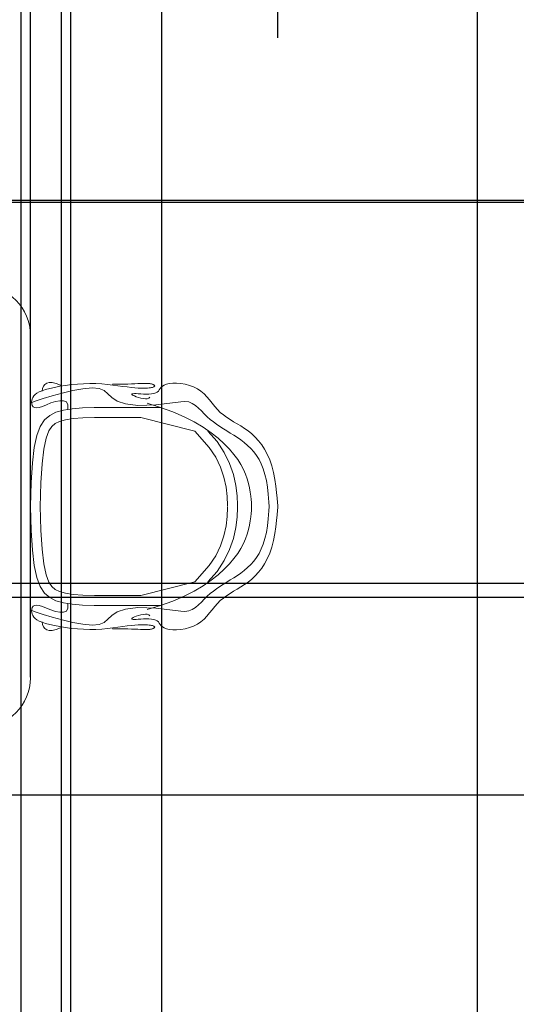
# Model space of a CAD drawing. Units: inches. Extents: x 1454 to 2136, y 626 to 1213.
# Tile 17 of 23: x 1701 to 1741, y 1062 to 1141. Entities that reach past the tile are written whole.
import ezdxf

# ---------------------------------------------------------------- set-up
doc = ezdxf.new("R2010")
doc.units = ezdxf.units.IN
doc.header["$MEASUREMENT"] = 0
for name, color, linetype, lineweight in [('A-ANNO-DIMS', 2, 'Continuous', 18), ('A-FURN-PATT', 252, 'Continuous', 13), ('conference', 41, 'Continuous', 18)]:
    doc.layers.add(name, color=color, linetype=linetype, lineweight=lineweight)
doc.styles.get("Standard").update_dxf_attribs({"font": 'arial.ttf'})
doc.dimstyles.get("Standard").update_dxf_attribs({"dimtxt": 4, "dimasz": 0.18, "dimexe": 0.18, "dimexo": 0.0625, "dimgap": 0.09, "dimtad": 0, "dimtih": 1, "dimtoh": 1, "dimdec": 0, "dimrnd": 6, "dimzin": 0, "dimdsep": 46, "dimlunit": 3, "dimtxsty": 'Standard', "dimcen": 0.09, "dimadec": 0, "dimazin": 0, "dimtfac": 1, "dimtdec": 0, "dimtofl": 0, "dimtmove": 0, "dimatfit": 3, "dimfxl": 1, "dimtolj": 1, "dimtzin": 0, "dimarcsym": 0})

# ---------------------------------------------------------------- blocks, each defined once
blk = doc.blocks.new('ОГ52_на12персон_стол2800х900')
for p, q in [((1400, 179.3), (1400, -520.7)), ((1433.5, 81.2), (1429.7, 78.7)), ((1438.5, 82.4), (1433.5, 81.2)), ((1444.8, 82.3), (1438.5, 82.4)), ((1452.5, 80.6), (1444.8, 82.3)), ((1461.7, 77.3), (1452.5, 80.6)), ((1629.1, 80.6), (1624.7, 80.4)), ((1633, 80.7), (1629.1, 80.6)), ((1636.3, 80.7), (1633, 80.7)), ((1639.2, 80.6), (1636.3, 80.7)), ((1641.7, 80.4), (1639.2, 80.6)), ((1643.8, 80.2), (1641.7, 80.4)), ((1683.8, 80.4), (1690.9, 81.1)), ((1690.9, 81.1), (1698.8, 81.1)), ((1698.8, 81.1), (1707.3, 80.4)), ((1409.5, 58), (1413.2, 60.6)), ((1413.2, 60.6), (1417.9, 63.2)), ((1417.9, 63.2), (1423.8, 65.6)), ((1425, 70.5), (1423.8, 65)), ((1423.8, 65.6), (1431, 68)), ((1426.9, 75.1), (1425, 70.5)), ((1429.7, 78.7), (1426.9, 75.1)), ((1431, 68), (1439.6, 70.4)), ((1439.6, 70.4), (1449.3, 72.6)), ((1465.2, 60.9), (1444.5, 55.2)), ((1449.3, 72.6), (1460.1, 74.7)), ((1460.1, 74.7), (1471.6, 76.5)), ((1486.6, 66), (1465.2, 60.9)), ((1471.6, 76.5), (1483.7, 78.1)), ((1483.7, 78.1), (1496.2, 79.3)), ((1507.4, 69.8), (1486.6, 66)), ((1496.2, 79.3), (1508.8, 80.1)), ((1526, 71.6), (1507.4, 69.8)), ((1508.8, 80.1), (1521.4, 80.4)), ((1521.4, 80.4), (1533.8, 80.2)), ((1540.7, 70.5), (1526, 71.6)), ((1533.8, 80.2), (1545.8, 79.5)), ((1550.8, 66.2), (1540.7, 70.5)), ((1545.8, 79.5), (1557.4, 78.6)), ((1558.5, 59.6), (1550.8, 66.2)), ((1557.4, 78.6), (1568.5, 77.3)), ((1579.5, 79.2), (1567.8, 79.4)), ((1568.5, 77.3), (1579, 76)), ((1579, 76), (1588.9, 74.6)), ((1589.9, 79.2), (1579.5, 79.2)), ((1588.9, 74.6), (1598, 73.4)), ((1598.9, 79.4), (1589.9, 79.2)), ((1598, 73.4), (1606.3, 72.3)), ((1606.8, 79.6), (1598.9, 79.4)), ((1606.3, 72.3), (1613.7, 71.5)), ((1613.7, 79.9), (1606.8, 79.6)), ((1619.6, 80.2), (1613.7, 79.9)), ((1613.7, 71.5), (1620.3, 71)), ((1624.7, 80.4), (1619.6, 80.2)), ((1620.3, 71), (1626.1, 70.7)), ((1626.1, 70.7), (1631.2, 70.7)), ((1631.2, 70.7), (1635.6, 70.7)), ((1635.6, 70.7), (1639.4, 71)), ((1639.4, 71), (1642.6, 71.3)), ((1642.6, 71.3), (1645.3, 71.7)), ((1645.6, 79.9), (1643.8, 80.2)), ((1645.3, 71.7), (1647.6, 72.1)), ((1647.2, 79.6), (1645.6, 79.9)), ((1648.6, 79.2), (1647.2, 79.6)), ((1647.6, 72.1), (1649.5, 72.6)), ((1649.8, 78.9), (1648.6, 79.2)), ((1649.5, 72.6), (1651, 73.1)), ((1650.9, 78.4), (1649.8, 78.9)), ((1651.8, 78), (1650.9, 78.4)), ((1651, 73.1), (1652.2, 73.6)), ((1652.6, 77.6), (1651.8, 78)), ((1652.2, 73.6), (1653, 74.1)), ((1652.2, 59.9), (1656.2, 61.1)), ((1653.2, 77.1), (1652.6, 77.6)), ((1653, 74.1), (1653.6, 74.6)), ((1653.6, 76.6), (1653.2, 77.1)), ((1653.9, 76.2), (1653.6, 76.6)), ((1653.6, 74.6), (1653.9, 75.1)), ((1654, 75.6), (1653.9, 76.2)), ((1653.9, 75.1), (1654, 75.6)), ((1656.2, 61.1), (1659.2, 62.9)), ((1659.2, 62.9), (1661.5, 65)), ((1661.5, 65), (1663.4, 67.5)), ((1663.4, 67.5), (1665.3, 70.1)), ((1665.3, 70.1), (1667.4, 72.7)), ((1667.4, 72.7), (1669.9, 75.2)), ((1669.9, 75.2), (1673.4, 77.4)), ((1673.4, 77.4), (1677.9, 79.2)), ((1677.9, 79.2), (1683.8, 80.4)), ((1707.3, 80.4), (1716.1, 78.9)), ((1716.1, 78.9), (1724.9, 76.7)), ((1724.9, 76.7), (1733.4, 73.6)), ((1733.4, 73.6), (1741.3, 69.7)), ((1741.3, 69.7), (1748.4, 64.9)), ((1748.4, 64.9), (1754.8, 59.3)), ((1402.5, 42.3), (1402.8, 45.8)), ((1402.9, 38.8), (1402.5, 42.3)), ((1411.6, 44.9), (1402.6, 41.8)), ((1402.8, 45.8), (1403.5, 49.1)), ((1403.5, 49.1), (1404.8, 52.2)), ((1404.8, 52.2), (1406.7, 55.2)), ((1406.7, 55.2), (1409.5, 58)), ((1426.1, 49.6), (1411.6, 44.9)), ((1444.5, 55.2), (1426.1, 49.6)), ((1432.7, 37.2), (1441.6, 40.7)), ((1441.6, 40.7), (1451, 43.6)), ((1451, 43.6), (1460, 45.4)), ((1460, 45.4), (1467.8, 45.4)), ((1467.8, 45.4), (1473.6, 42.8)), ((1473.6, 42.8), (1476.8, 37.1)), ((1566.4, 51.9), (1558.5, 59.6)), ((1577.3, 44.6), (1566.4, 51.9)), ((1594.1, 38.7), (1577.3, 44.6)), ((1607.1, 58.9), (1608, 59.4)), ((1607.1, 58.2), (1607.1, 58.9)), ((1608, 57.4), (1607.1, 58.2)), ((1608, 59.4), (1609.8, 59.7)), ((1609.9, 56.3), (1608, 57.4)), ((1609.8, 59.7), (1612.5, 59.9)), ((1612.7, 55), (1609.9, 56.3)), ((1612.5, 59.9), (1616.1, 59.8)), ((1616.4, 53.5), (1612.7, 55)), ((1616.1, 59.8), (1620.5, 59.6)), ((1620.8, 52), (1616.4, 53.5)), ((1620.5, 59.6), (1625.5, 59.3)), ((1625.5, 50.7), (1620.8, 52)), ((1625.5, 59.3), (1631, 59)), ((1630.3, 49.7), (1625.5, 50.7)), ((1634.9, 49.2), (1630.3, 49.7)), ((1631, 59), (1636.6, 58.9)), ((1638.9, 49.4), (1634.9, 49.2)), ((1636.6, 58.9), (1642.2, 58.9)), ((1642.1, 50.6), (1638.9, 49.4)), ((1644.1, 52.8), (1642.1, 50.6)), ((1642.2, 58.9), (1647.5, 59.2)), ((1647.5, 59.2), (1652.2, 59.9)), ((1707.2, 43.1), (1656.2, 36.7)), ((1707.2, 43.1), (1715.9, 43.9)), ((1715.9, 43.9), (1723.6, 42.7)), ((1723.6, 42.7), (1730.7, 39.8)), ((1754.8, 59.3), (1760.7, 53.2)), ((1760.7, 53.2), (1766.3, 46.8)), ((1766.3, 46.8), (1771.6, 40.2)), ((1403.9, 35.6), (1402.9, 38.8)), ((1405.8, 33), (1403.9, 35.6)), ((1408.7, 31.2), (1405.8, 33)), ((1412.8, 30.6), (1408.7, 31.2)), ((1418.1, 31.4), (1412.8, 30.6)), ((1424.9, 33.8), (1418.1, 31.4)), ((1424.9, 33.8), (1432.7, 37.2)), ((1452.2, 21.8), (1439.4, 15.4)), ((1467.4, 26.2), (1452.2, 21.8)), ((1485.4, 29), (1467.4, 26.2)), ((1476.8, 37.1), (1476.4, 27.6)), ((1506.3, 30.5), (1485.4, 29)), ((1530.4, 31.2), (1506.3, 30.5)), ((1558.2, 31.3), (1530.4, 31.2)), ((1589.9, 31.2), (1558.2, 31.3)), ((1625.8, 31.2), (1589.9, 31.2)), ((1619.4, 35.7), (1594.1, 38.7)), ((1656.2, 36.7), (1619.4, 35.7)), ((1666.1, 31.7), (1625.8, 31.2)), ((1638.3, 40), (1666.1, 31.7)), ((1666.1, 31.7), (1691.4, 22.5)), ((1691.4, 22.5), (1714.2, 12.5)), ((1730.7, 39.8), (1737.3, 35.6)), ((1737.3, 35.6), (1743.5, 30.4)), ((1743.5, 30.4), (1749.4, 24.7)), ((1749.4, 24.7), (1755.3, 18.6)), ((1771.6, 40.2), (1776.9, 33.7)), ((1776.9, 33.7), (1782.4, 27.4)), ((1782.4, 27.4), (1788.1, 21.5)), ((1788.1, 21.5), (1794.4, 16.2)), ((1428.7, 6.1), (1420.1, -7.2)), ((1439.4, 15.4), (1428.7, 6.1)), ((1459.5, 3.1), (1450.6, -1.3)), ((1471.7, 6.6), (1459.5, 3.1)), ((1487.6, 9.1), (1471.7, 6.6)), ((1507.3, 10.5), (1487.6, 9.1)), ((1530.8, 11.2), (1507.3, 10.5)), ((1558.2, 11.3), (1530.8, 11.2)), ((1589.9, 11.2), (1558.2, 11.3)), ((1625.9, 11.2), (1589.9, 11.2)), ((1735.7, -17.1), (1625.9, 11.2)), ((1714.2, 12.5), (1734.8, 2)), ((1734.8, 2), (1753.1, -8.9)), ((1755.3, 18.6), (1761.3, 12.7)), ((1761.3, 12.7), (1767.5, 7.2)), ((1767.5, 7.2), (1773.9, 2.1)), ((1773.9, 2.1), (1780.6, -2.8)), ((1794.4, 16.2), (1801, 11.4)), ((1801, 11.4), (1808, 6.9)), ((1808, 6.9), (1815.2, 2.5)), ((1815.2, 2.5), (1822.6, -1.8)), ((1420.1, -7.2), (1413.2, -25.6)), ((1438, -16.3), (1432.5, -31.2)), ((1444, -7.1), (1438, -16.3)), ((1450.6, -1.3), (1444, -7.1)), ((1735.7, -17.1), (1765.6, -50.4)), ((1753.1, -8.9), (1769.4, -20.1)), ((1762.3, -16.7), (1781.4, -38.1)), ((1769.4, -20.1), (1783.7, -31.3)), ((1780.6, -2.8), (1787.4, -7.4)), ((1787.4, -7.4), (1794.3, -11.8)), ((1794.3, -11.8), (1801.4, -16.3)), ((1801.4, -16.3), (1808.5, -20.7)), ((1822.6, -1.8), (1830.1, -6.3)), ((1830.1, -6.3), (1837.6, -11.1)), ((1837.6, -11.1), (1845, -16.4)), ((1845, -16.4), (1852.3, -22.3)), ((1413.2, -25.6), (1408, -50.1)), ((1432.5, -31.2), (1427.7, -53.4)), ((1781.4, -38.1), (1796.2, -60.3)), ((1783.7, -31.3), (1796.1, -42.5)), ((1808.5, -20.7), (1815.7, -25.2)), ((1815.7, -25.2), (1822.9, -29.9)), ((1822.9, -29.9), (1830, -34.9)), ((1830, -34.9), (1837, -40.2)), ((1837, -40.2), (1843.8, -45.9)), ((1852.3, -22.3), (1859.4, -29)), ((1859.4, -29), (1866.2, -36.3)), ((1866.2, -36.3), (1872.7, -44.6)), ((1408, -50.1), (1404.2, -81.7)), ((1427.7, -53.4), (1424.1, -83.6)), ((1765.6, -50.4), (1778.8, -70.2)), ((1796.1, -42.5), (1806.8, -53.5)), ((1796.2, -60.3), (1807.2, -82.9)), ((1806.8, -53.5), (1816, -64.2)), ((1843.8, -45.9), (1850.3, -52.2)), ((1850.3, -52.2), (1856.4, -59)), ((1856.4, -59), (1862.1, -66.5)), ((1872.7, -44.6), (1878.7, -53.8)), ((1878.7, -53.8), (1884.1, -64)), ((1778.8, -70.2), (1788.7, -90.5)), ((1816, -64.2), (1823.7, -74.7)), ((1823.7, -74.7), (1830.1, -84.9)), ((1862.1, -66.5), (1867.3, -74.8)), ((1867.3, -74.8), (1871.9, -83.9)), ((1884.1, -64), (1889, -75.2)), ((1889, -75.2), (1893.2, -87.7)), ((1404.2, -81.7), (1401.6, -121.6)), ((1424.1, -83.6), (1421.5, -122.5)), ((1788.7, -90.5), (1795.5, -110.8)), ((1807.2, -82.9), (1814.8, -105.5)), ((1830.1, -84.9), (1835.3, -94.9)), ((1835.3, -94.9), (1839.6, -104.7)), ((1871.9, -83.9), (1875.9, -94)), ((1875.9, -94), (1879.3, -105.1)), ((1893.2, -87.7), (1896.7, -101.2)), ((1795.5, -110.8), (1800, -130.9)), ((1814.8, -105.5), (1819.7, -127.5)), ((1839.6, -104.7), (1843, -114.3)), ((1843, -114.3), (1845.6, -123.7)), ((1879.3, -105.1), (1882.2, -117.4)), ((1882.2, -117.4), (1884.5, -130.9)), ((1896.7, -101.2), (1899.4, -115.3)), ((1899.4, -115.3), (1901.6, -129.2)), ((1401.6, -121.6), (1400, -170.7)), ((1421.5, -122.5), (1420, -171.3)), ((1800, -130.9), (1802.3, -150.3)), ((1819.7, -127.5), (1822.3, -148.6)), ((1845.6, -123.7), (1847.7, -132.7)), ((1847.7, -132.7), (1849.2, -141.4)), ((1884.5, -130.9), (1886.2, -145.8)), ((1901.6, -129.2), (1903.2, -142.1)), ((1802.3, -150.3), (1803.1, -168.6)), ((1822.3, -148.6), (1823.1, -168.3)), ((1849.2, -141.4), (1850.3, -149.3)), ((1850.3, -149.3), (1851, -156.4)), ((1851, -156.4), (1851.5, -162.3)), ((1886.2, -145.8), (1887.4, -162.1)), ((1903.2, -142.1), (1904.4, -153.5)), ((1904.4, -153.5), (1905.1, -162.5)), ((1401.6, -219.8), (1400, -170.7)), ((1421.5, -218.8), (1420, -170)), ((1802.3, -191.1), (1803.1, -172.8)), ((1803.1, -168.6), (1803.1, -170.3)), ((1803.1, -172.8), (1803.1, -171.1)), ((1822.3, -192.7), (1823.1, -173)), ((1823.1, -168.3), (1823.1, -170.7)), ((1823.1, -173), (1823.1, -170.7)), ((1851, -185), (1851.5, -179.1)), ((1851.5, -162.3), (1851.7, -166.8)), ((1851.5, -179.1), (1851.7, -174.6)), ((1851.7, -166.8), (1851.8, -169.6)), ((1851.7, -174.6), (1851.8, -171.7)), ((1851.8, -169.6), (1851.8, -170.7)), ((1851.8, -171.7), (1851.8, -170.7)), ((1886.2, -195.6), (1887.4, -179.3)), ((1887.4, -162.1), (1887.8, -170.7)), ((1887.4, -179.3), (1887.8, -170.7)), ((1904.4, -187.9), (1905.1, -178.9)), ((1905.1, -162.5), (1905.5, -168.5)), ((1905.1, -178.9), (1905.5, -172.9)), ((1905.5, -168.5), (1905.7, -170.7)), ((1905.5, -172.9), (1905.7, -170.7)), ((1800, -210.5), (1802.3, -191.1)), ((1819.7, -213.8), (1822.3, -192.7)), ((1847.7, -208.6), (1849.2, -200)), ((1849.2, -200), (1850.3, -192)), ((1850.3, -192), (1851, -185)), ((1884.5, -210.5), (1886.2, -195.6)), ((1901.6, -212.2), (1903.2, -199.2)), ((1903.2, -199.2), (1904.4, -187.9)), ((1404.2, -259.6), (1401.6, -219.8)), ((1424.1, -257.8), (1421.5, -218.8)), ((1795.5, -230.5), (1800, -210.5)), ((1814.8, -235.9), (1819.7, -213.8)), ((1843, -227), (1845.6, -217.7)), ((1845.6, -217.7), (1847.7, -208.6)), ((1882.2, -224), (1884.5, -210.5)), ((1899.4, -226.1), (1901.6, -212.2)), ((1788.7, -250.9), (1795.5, -230.5)), ((1807.2, -258.5), (1814.8, -235.9)), ((1835.3, -246.4), (1839.6, -236.6)), ((1839.6, -236.6), (1843, -227)), ((1875.9, -247.3), (1879.3, -236.2)), ((1879.3, -236.2), (1882.2, -224)), ((1893.2, -253.7), (1896.7, -240.1)), ((1896.7, -240.1), (1899.4, -226.1)), ((1408, -291.3), (1404.2, -259.6)), ((1427.7, -288), (1424.1, -257.8)), ((1778.8, -271.1), (1788.7, -250.9)), ((1796.2, -281.1), (1807.2, -258.5)), ((1823.7, -266.7), (1830.1, -256.4)), ((1830.1, -256.4), (1835.3, -246.4)), ((1867.3, -266.5), (1871.9, -257.4)), ((1871.9, -257.4), (1875.9, -247.3)), ((1889, -266.1), (1893.2, -253.7)), ((1765.6, -291), (1778.8, -271.1)), ((1781.4, -303.3), (1796.2, -281.1)), ((1806.8, -287.9), (1816, -277.2)), ((1816, -277.2), (1823.7, -266.7)), ((1856.4, -282.3), (1862.1, -274.8)), ((1862.1, -274.8), (1867.3, -266.5)), ((1878.7, -287.6), (1884.1, -277.4)), ((1884.1, -277.4), (1889, -266.1)), ((1413.2, -315.8), (1408, -291.3)), ((1432.5, -310.2), (1427.7, -288)), ((1735.7, -324.3), (1765.6, -291)), ((1783.7, -310), (1796.1, -298.9)), ((1796.1, -298.9), (1806.8, -287.9)), ((1830, -306.5), (1837, -301.2)), ((1837, -301.2), (1843.8, -295.4)), ((1843.8, -295.4), (1850.3, -289.2)), ((1850.3, -289.2), (1856.4, -282.3)), ((1866.2, -305), (1872.7, -296.8)), ((1872.7, -296.8), (1878.7, -287.6)), ((1420.1, -334.1), (1413.2, -315.8)), ((1438, -325.1), (1432.5, -310.2)), ((1753.1, -332.5), (1769.4, -321.3)), ((1762.3, -324.6), (1781.4, -303.3)), ((1769.4, -321.3), (1783.7, -310)), ((1801.4, -325.1), (1808.5, -320.7)), ((1808.5, -320.7), (1815.7, -316.1)), ((1815.7, -316.1), (1822.9, -311.4)), ((1822.9, -311.4), (1830, -306.5)), ((1845, -324.9), (1852.3, -319)), ((1852.3, -319), (1859.4, -312.4)), ((1859.4, -312.4), (1866.2, -305)), ((1428.7, -347.5), (1420.1, -334.1)), ((1444, -334.2), (1438, -325.1)), ((1450.6, -340), (1444, -334.2)), ((1459.5, -344.4), (1450.6, -340)), ((1735.7, -324.3), (1625.9, -352.6)), ((1734.8, -343.4), (1753.1, -332.5)), ((1773.9, -343.4), (1780.6, -338.6)), ((1780.6, -338.6), (1787.4, -334)), ((1787.4, -334), (1794.3, -329.5)), ((1794.3, -329.5), (1801.4, -325.1)), ((1815.2, -343.9), (1822.6, -339.5)), ((1822.6, -339.5), (1830.1, -335)), ((1830.1, -335), (1837.6, -330.2)), ((1837.6, -330.2), (1845, -324.9)), ((1439.4, -356.8), (1428.7, -347.5)), ((1452.2, -363.2), (1439.4, -356.8)), ((1471.7, -348), (1459.5, -344.4)), ((1487.6, -350.4), (1471.7, -348)), ((1507.3, -351.9), (1487.6, -350.4)), ((1530.8, -352.6), (1507.3, -351.9)), ((1558.2, -352.7), (1530.8, -352.6)), ((1589.9, -352.6), (1558.2, -352.7)), ((1625.9, -352.6), (1589.9, -352.6)), ((1691.4, -363.8), (1714.2, -353.9)), ((1714.2, -353.9), (1734.8, -343.4)), ((1749.4, -366), (1755.3, -360)), ((1755.3, -360), (1761.3, -354.1)), ((1761.3, -354.1), (1767.5, -348.6)), ((1767.5, -348.6), (1773.9, -343.4)), ((1788.1, -362.9), (1794.4, -357.6)), ((1794.4, -357.6), (1801, -352.8)), ((1801, -352.8), (1808, -348.2)), ((1808, -348.2), (1815.2, -343.9)), ((1402.9, -380.1), (1402.5, -383.6)), ((1403.9, -376.9), (1402.9, -380.1)), ((1405.8, -374.3), (1403.9, -376.9)), ((1408.7, -372.6), (1405.8, -374.3)), ((1412.8, -372), (1408.7, -372.6)), ((1418.1, -372.7), (1412.8, -372)), ((1424.9, -375.1), (1418.1, -372.7)), ((1424.9, -375.1), (1432.7, -378.5)), ((1432.7, -378.5), (1441.6, -382)), ((1467.4, -367.5), (1452.2, -363.2)), ((1485.4, -370.3), (1467.4, -367.5)), ((1473.6, -384.2), (1476.8, -378.4)), ((1476.8, -378.4), (1476.4, -368.9)), ((1506.3, -371.9), (1485.4, -370.3)), ((1530.4, -372.6), (1506.3, -371.9)), ((1558.2, -372.7), (1530.4, -372.6)), ((1589.9, -372.6), (1558.2, -372.7)), ((1594.1, -380.1), (1577.3, -385.9)), ((1625.8, -372.6), (1589.9, -372.6)), ((1619.4, -377.1), (1594.1, -380.1)), ((1656.2, -378.1), (1619.4, -377.1)), ((1666.1, -373), (1625.8, -372.6)), ((1638.3, -381.3), (1666.1, -373)), ((1707.2, -384.5), (1656.2, -378.1)), ((1666.1, -373), (1691.4, -363.8)), ((1723.6, -384), (1730.7, -381.1)), ((1730.7, -381.1), (1737.3, -376.9)), ((1737.3, -376.9), (1743.5, -371.8)), ((1743.5, -371.8), (1749.4, -366)), ((1766.3, -388.1), (1771.6, -381.6)), ((1771.6, -381.6), (1776.9, -375)), ((1776.9, -375), (1782.4, -368.7)), ((1782.4, -368.7), (1788.1, -362.9)), ((1402.5, -383.6), (1402.8, -387.1)), ((1411.6, -386.3), (1402.6, -383.2)), ((1402.8, -387.1), (1403.5, -390.5)), ((1403.5, -390.5), (1404.8, -393.6)), ((1404.8, -393.6), (1406.7, -396.6)), ((1406.7, -396.6), (1409.5, -399.3)), ((1409.5, -399.3), (1413.2, -402)), ((1426.1, -391), (1411.6, -386.3)), ((1413.2, -402), (1417.9, -404.5)), ((1444.5, -396.5), (1426.1, -391)), ((1441.6, -382), (1451, -385)), ((1465.2, -402.3), (1444.5, -396.5)), ((1451, -385), (1460, -386.8)), ((1460, -386.8), (1467.8, -386.7)), ((1467.8, -386.7), (1473.6, -384.2)), ((1558.5, -400.9), (1550.8, -407.5)), ((1566.4, -393.3), (1558.5, -400.9)), ((1577.3, -385.9), (1566.4, -393.3)), ((1608, -398.7), (1607.1, -399.6)), ((1607.1, -399.6), (1607.1, -400.3)), ((1607.1, -400.3), (1608, -400.8)), ((1609.9, -397.6), (1608, -398.7)), ((1608, -400.8), (1609.8, -401.1)), ((1609.8, -401.1), (1612.5, -401.2)), ((1612.7, -396.3), (1609.9, -397.6)), ((1612.5, -401.2), (1616.1, -401.2)), ((1616.4, -394.9), (1612.7, -396.3)), ((1616.1, -401.2), (1620.5, -401)), ((1620.8, -393.4), (1616.4, -394.9)), ((1620.5, -401), (1625.5, -400.7)), ((1625.5, -392), (1620.8, -393.4)), ((1630.3, -391.1), (1625.5, -392)), ((1625.5, -400.7), (1631, -400.4)), ((1634.9, -390.6), (1630.3, -391.1)), ((1631, -400.4), (1636.6, -400.2)), ((1638.9, -390.8), (1634.9, -390.6)), ((1636.6, -400.2), (1642.2, -400.3)), ((1642.1, -391.9), (1638.9, -390.8)), ((1644.1, -394.1), (1642.1, -391.9)), ((1642.2, -400.3), (1647.5, -400.6)), ((1647.5, -400.6), (1652.2, -401.3)), ((1652.2, -401.3), (1656.2, -402.5)), ((1707.2, -384.5), (1715.9, -385.3)), ((1715.9, -385.3), (1723.6, -384)), ((1748.4, -406.2), (1754.8, -400.7)), ((1754.8, -400.7), (1760.7, -394.6)), ((1760.7, -394.6), (1766.3, -388.1)), ((1417.9, -404.5), (1423.8, -407)), ((1425, -411.9), (1423.8, -406.4)), ((1423.8, -407), (1431, -409.4)), ((1426.9, -416.5), (1425, -411.9)), ((1429.7, -420.1), (1426.9, -416.5)), ((1433.5, -422.6), (1429.7, -420.1)), ((1431, -409.4), (1439.6, -411.7)), ((1439.6, -411.7), (1449.3, -414)), ((1452.5, -422), (1444.8, -423.7)), ((1449.3, -414), (1460.1, -416)), ((1461.7, -418.7), (1452.5, -422)), ((1460.1, -416), (1471.6, -417.9)), ((1486.6, -407.4), (1465.2, -402.3)), ((1471.6, -417.9), (1483.7, -419.5)), ((1483.7, -419.5), (1496.2, -420.7)), ((1507.4, -411.2), (1486.6, -407.4)), ((1496.2, -420.7), (1508.8, -421.5)), ((1526, -412.9), (1507.4, -411.2)), ((1508.8, -421.5), (1521.4, -421.8)), ((1521.4, -421.8), (1533.8, -421.6)), ((1540.7, -411.8), (1526, -412.9)), ((1533.8, -421.6), (1545.8, -420.9)), ((1550.8, -407.5), (1540.7, -411.8)), ((1545.8, -420.9), (1557.4, -419.9)), ((1557.4, -419.9), (1568.5, -418.7)), ((1579.5, -420.6), (1567.8, -420.7)), ((1568.5, -418.7), (1579, -417.4)), ((1579, -417.4), (1588.9, -416)), ((1589.9, -420.6), (1579.5, -420.6)), ((1588.9, -416), (1598, -414.7)), ((1598.9, -420.7), (1589.9, -420.6)), ((1598, -414.7), (1606.3, -413.7)), ((1606.8, -421), (1598.9, -420.7)), ((1606.3, -413.7), (1613.7, -412.9)), ((1613.7, -421.2), (1606.8, -421)), ((1613.7, -412.9), (1620.3, -412.4)), ((1619.6, -421.5), (1613.7, -421.2)), ((1624.7, -421.8), (1619.6, -421.5)), ((1620.3, -412.4), (1626.1, -412.1)), ((1629.1, -422), (1624.7, -421.8)), ((1626.1, -412.1), (1631.2, -412)), ((1633, -422), (1629.1, -422)), ((1631.2, -412), (1635.6, -412.1)), ((1636.3, -422), (1633, -422)), ((1635.6, -412.1), (1639.4, -412.3)), ((1639.2, -422), (1636.3, -422)), ((1641.7, -421.8), (1639.2, -422)), ((1639.4, -412.3), (1642.6, -412.7)), ((1643.8, -421.6), (1641.7, -421.8)), ((1642.6, -412.7), (1645.3, -413)), ((1645.6, -421.3), (1643.8, -421.6)), ((1645.3, -413), (1647.6, -413.5)), ((1647.2, -421), (1645.6, -421.3)), ((1648.6, -420.6), (1647.2, -421)), ((1647.6, -413.5), (1649.5, -413.9)), ((1649.8, -420.2), (1648.6, -420.6)), ((1649.5, -413.9), (1651, -414.4)), ((1650.9, -419.8), (1649.8, -420.2)), ((1651.8, -419.4), (1650.9, -419.8)), ((1651, -414.4), (1652.2, -414.9)), ((1652.6, -418.9), (1651.8, -419.4)), ((1652.2, -414.9), (1653, -415.4)), ((1653.2, -418.5), (1652.6, -418.9)), ((1653, -415.4), (1653.6, -416)), ((1653.6, -418), (1653.2, -418.5)), ((1653.6, -416), (1653.9, -416.5)), ((1653.9, -417.5), (1653.6, -418)), ((1653.9, -416.5), (1654, -417)), ((1654, -417), (1653.9, -417.5)), ((1656.2, -402.5), (1659.2, -404.2)), ((1659.2, -404.2), (1661.5, -406.4)), ((1661.5, -406.4), (1663.4, -408.8)), ((1663.4, -408.8), (1665.3, -411.4)), ((1665.3, -411.4), (1667.4, -414.1)), ((1667.4, -414.1), (1669.9, -416.5)), ((1669.9, -416.5), (1673.4, -418.7)), ((1673.4, -418.7), (1677.9, -420.5)), ((1677.9, -420.5), (1683.8, -421.8)), ((1683.8, -421.8), (1690.9, -422.4)), ((1698.8, -422.4), (1707.3, -421.7)), ((1707.3, -421.7), (1716.1, -420.3)), ((1716.1, -420.3), (1724.9, -418)), ((1724.9, -418), (1733.4, -415)), ((1733.4, -415), (1741.3, -411)), ((1741.3, -411), (1748.4, -406.2)), ((1438.5, -423.8), (1433.5, -422.6)), ((1444.8, -423.7), (1438.5, -423.8)), ((1690.9, -422.4), (1698.8, -422.4))]:
    blk.add_line(p, q)
for centre, start, end in [((1300, 179.3), 0, 90), ((1300, -520.7), 270, 0)]:
    blk.add_arc(centre, 100, start, end)
blk = doc.blocks.new('*D23')
at = {"layer": 'A-ANNO-DIMS', "color": 0, "lineweight": -2, "transparency": 16777216}
for p, q in [((1571.674, 1139.532), (1571.674, 1162.157)), ((1721.725, 1139.532), (1721.725, 1162.157)), ((1571.854, 1161.977), (1615.675, 1161.977)), ((1721.545, 1161.977), (1677.724, 1161.977))]:
    blk.add_line(p, q, dxfattribs=at)
at = {"layer": 'A-ANNO-DIMS', "color": 0, "transparency": 16777216}
for points in [[(1571.854, 1162.007), (1571.854, 1161.947), (1571.674, 1161.977)], [(1721.545, 1162.007), (1721.545, 1161.947), (1721.725, 1161.977)]]:
    blk.add_solid(points, dxfattribs=at)
at = {"layer": 'Defpoints', "color": 0, "transparency": 16777216}
for p in [(1721.725, 1161.977), (1571.674, 1139.469), (1721.725, 1139.469)]:
    blk.add_point(p, dxfattribs=at)
at = {"layer": 'A-ANNO-DIMS', "color": 0, "transparency": 16777216, "insert": (1646.7, 1161.977), "char_height": 4, "attachment_point": 5}
blk.add_mtext('\\A1;CONFERENCE SET 150', dxfattribs=at)
blk = doc.blocks.new('*D33')
at = {"layer": 'A-ANNO-DIMS', "color": 0, "lineweight": -2, "transparency": 16777216}
for p, q in [((2032.494, 1126.282), (1462.374, 1126.282)), ((1462.554, 1126.102), (1462.554, 1056.381)), ((1462.554, 982.462), (1462.554, 1052.184)), ((2032.494, 982.282), (1462.374, 982.282))]:
    blk.add_line(p, q, dxfattribs=at)
at = {"layer": 'A-ANNO-DIMS', "color": 0, "transparency": 16777216}
for points in [[(1462.524, 1126.102), (1462.584, 1126.102), (1462.554, 1126.282)], [(1462.524, 982.462), (1462.584, 982.462), (1462.554, 982.282)]]:
    blk.add_solid(points, dxfattribs=at)
at = {"layer": 'Defpoints', "color": 0, "transparency": 16777216}
for p in [(1462.554, 1126.282), (2032.556, 1126.282), (2032.556, 982.282)]:
    blk.add_point(p, dxfattribs=at)
at = {"layer": 'A-ANNO-DIMS', "color": 0, "transparency": 16777216, "insert": (1462.554, 1054.282), "char_height": 4, "attachment_point": 5}
blk.add_mtext('\\A1;144', dxfattribs=at)
blk = doc.blocks.new('*D44')
at = {"layer": 'A-ANNO-DIMS', "color": 0, "lineweight": -2, "transparency": 16777216}
for p, q in [((1701.076, 909.11), (1701.076, 1210.464)), ((1701.256, 1210.284), (1784.958, 1210.284)), ((1885.07, 1210.284), (1801.368, 1210.284)), ((1885.25, 909.11), (1885.25, 1210.464))]:
    blk.add_line(p, q, dxfattribs=at)
at = {"layer": 'A-ANNO-DIMS', "color": 0, "transparency": 16777216}
for points in [[(1701.256, 1210.314), (1701.256, 1210.254), (1701.076, 1210.284)], [(1885.07, 1210.314), (1885.07, 1210.254), (1885.25, 1210.284)]]:
    blk.add_solid(points, dxfattribs=at)
at = {"layer": 'Defpoints', "color": 0, "transparency": 16777216}
for p in [(1885.25, 1210.284), (1701.076, 909.048), (1885.25, 909.048)]:
    blk.add_point(p, dxfattribs=at)
at = {"layer": 'A-ANNO-DIMS', "color": 0, "transparency": 16777216, "insert": (1793.163, 1210.284), "char_height": 4, "attachment_point": 5}
blk.add_mtext('\\A1;184.17', dxfattribs=at)
blk = doc.blocks.new('*D45')
at = {"layer": 'A-ANNO-DIMS', "color": 0, "lineweight": -2, "transparency": 16777216}
for p, q in [((1654.556, 913.345), (1654.556, 1210.464)), ((1654.736, 1210.284), (1670.917, 1210.284)), ((1700.896, 1210.284), (1684.715, 1210.284)), ((1701.076, 909.11), (1701.076, 1210.464))]:
    blk.add_line(p, q, dxfattribs=at)
at = {"layer": 'A-ANNO-DIMS', "color": 0, "transparency": 16777216}
for points in [[(1654.736, 1210.314), (1654.736, 1210.254), (1654.556, 1210.284)], [(1700.896, 1210.314), (1700.896, 1210.254), (1701.076, 1210.284)]]:
    blk.add_solid(points, dxfattribs=at)
at = {"layer": 'Defpoints', "color": 0, "transparency": 16777216}
for p in [(1701.076, 1210.284), (1654.556, 913.282), (1701.076, 909.048)]:
    blk.add_point(p, dxfattribs=at)
at = {"layer": 'A-ANNO-DIMS', "color": 0, "transparency": 16777216, "insert": (1677.816, 1210.284), "char_height": 4, "attachment_point": 5}
blk.add_mtext('\\A1;46.52', dxfattribs=at)
blk = doc.blocks.new('*D54')
at = {"layer": 'A-ANNO-DIMS', "color": 0, "lineweight": -2, "transparency": 16777216}
for p, q in [((1879.494, 1126.282), (1462.374, 1126.282)), ((1462.554, 1126.102), (1462.554, 1078.915)), ((1462.554, 1027.462), (1462.554, 1074.65)), ((1879.494, 1027.282), (1462.374, 1027.282))]:
    blk.add_line(p, q, dxfattribs=at)
at = {"layer": 'A-ANNO-DIMS', "color": 0, "transparency": 16777216}
for points in [[(1462.524, 1126.102), (1462.584, 1126.102), (1462.554, 1126.282)], [(1462.524, 1027.462), (1462.584, 1027.462), (1462.554, 1027.282)]]:
    blk.add_solid(points, dxfattribs=at)
at = {"layer": 'Defpoints', "color": 0, "transparency": 16777216}
for p in [(1879.556, 1126.282), (1462.554, 1027.282), (1879.556, 1027.282)]:
    blk.add_point(p, dxfattribs=at)
at = {"layer": 'A-ANNO-DIMS', "color": 0, "transparency": 16777216, "insert": (1462.554, 1076.782), "char_height": 4, "attachment_point": 5}
blk.add_mtext('\\A1;99', dxfattribs=at)
blk = doc.blocks.new('*D68')
at = {"layer": 'A-ANNO-DIMS', "color": 0, "lineweight": -2, "transparency": 16777216}
for p, q in [((1659.724, 1027.329), (1659.724, 1210.464)), ((1659.904, 1210.284), (1675.092, 1210.284)), ((1704.128, 1210.284), (1688.939, 1210.284)), ((1704.308, 1027.329), (1704.308, 1210.464))]:
    blk.add_line(p, q, dxfattribs=at)
at = {"layer": 'A-ANNO-DIMS', "color": 0, "transparency": 16777216}
for points in [[(1659.904, 1210.314), (1659.904, 1210.254), (1659.724, 1210.284)], [(1704.128, 1210.314), (1704.128, 1210.254), (1704.308, 1210.284)]]:
    blk.add_solid(points, dxfattribs=at)
at = {"layer": 'Defpoints', "color": 0, "transparency": 16777216}
for p in [(1704.308, 1210.284), (1659.724, 1027.267), (1704.308, 1027.267)]:
    blk.add_point(p, dxfattribs=at)
at = {"layer": 'A-ANNO-DIMS', "color": 0, "transparency": 16777216, "insert": (1682.016, 1210.284), "char_height": 4, "attachment_point": 5}
blk.add_mtext('\\A1;44.58', dxfattribs=at)
blk = doc.blocks.new('*D70')
at = {"layer": 'A-ANNO-DIMS', "color": 0, "lineweight": -2, "transparency": 16777216}
for p, q in [((1811.166, 1094.525), (1462.374, 1094.525)), ((1462.554, 1094.345), (1462.554, 1088.71)), ((1462.554, 1078.811), (1462.554, 1084.445)), ((1811.166, 1078.631), (1462.374, 1078.631))]:
    blk.add_line(p, q, dxfattribs=at)
at = {"layer": 'A-ANNO-DIMS', "color": 0, "transparency": 16777216}
for points in [[(1462.524, 1094.345), (1462.584, 1094.345), (1462.554, 1094.525)], [(1462.524, 1078.811), (1462.584, 1078.811), (1462.554, 1078.631)]]:
    blk.add_solid(points, dxfattribs=at)
at = {"layer": 'Defpoints', "color": 0, "transparency": 16777216}
for p in [(1462.554, 1094.525), (1811.229, 1094.525), (1811.229, 1078.631)]:
    blk.add_point(p, dxfattribs=at)
at = {"layer": 'A-ANNO-DIMS', "color": 0, "transparency": 16777216, "insert": (1462.554, 1086.578), "char_height": 4, "attachment_point": 5}
blk.add_mtext('\\A1;15.894', dxfattribs=at)
blk = doc.blocks.new('*D71')
at = {"layer": 'A-ANNO-DIMS', "color": 0, "lineweight": -2, "transparency": 16777216}
for p, q in [((1712.389, 694.263), (1712.389, 1210.464)), ((1712.569, 1210.284), (1718.607, 1210.284)), ((1737.62, 1210.284), (1731.581, 1210.284)), ((1737.8, 694.263), (1737.8, 1210.464))]:
    blk.add_line(p, q, dxfattribs=at)
at = {"layer": 'A-ANNO-DIMS', "color": 0, "transparency": 16777216}
for points in [[(1712.569, 1210.314), (1712.569, 1210.254), (1712.389, 1210.284)], [(1737.62, 1210.314), (1737.62, 1210.254), (1737.8, 1210.284)]]:
    blk.add_solid(points, dxfattribs=at)
at = {"layer": 'Defpoints', "color": 0, "transparency": 16777216}
for p in [(1737.8, 1210.284), (1712.389, 694.201), (1737.8, 694.201)]:
    blk.add_point(p, dxfattribs=at)
at = {"layer": 'A-ANNO-DIMS', "color": 0, "transparency": 16777216, "insert": (1725.094, 1210.284), "char_height": 4, "attachment_point": 5}
blk.add_mtext('\\A1;25.41', dxfattribs=at)
blk = doc.blocks.new('*D73')
at = {"layer": 'A-ANNO-DIMS', "color": 0, "lineweight": -2, "transparency": 16777216}
for p, q in [((1985.096, 1126.439), (1462.374, 1126.439)), ((1462.554, 1126.259), (1462.554, 1113.178)), ((1462.554, 1095.83), (1462.554, 1108.911)), ((1966.644, 1095.65), (1462.374, 1095.65))]:
    blk.add_line(p, q, dxfattribs=at)
at = {"layer": 'A-ANNO-DIMS', "color": 0, "transparency": 16777216}
for points in [[(1462.524, 1126.259), (1462.584, 1126.259), (1462.554, 1126.439)], [(1462.524, 1095.83), (1462.584, 1095.83), (1462.554, 1095.65)]]:
    blk.add_solid(points, dxfattribs=at)
at = {"layer": 'Defpoints', "color": 0, "transparency": 16777216}
for p in [(1985.158, 1126.439), (1462.554, 1095.65), (1966.707, 1095.65)]:
    blk.add_point(p, dxfattribs=at)
at = {"layer": 'A-ANNO-DIMS', "color": 0, "transparency": 16777216, "insert": (1462.554, 1111.044), "char_height": 4, "attachment_point": 5}
blk.add_mtext('\\A1;30.79', dxfattribs=at)
blk = doc.blocks.new('*D76')
at = {"layer": 'A-ANNO-DIMS', "color": 0, "lineweight": -2, "transparency": 16777216}
for p, q in [((1962.644, 1095.65), (1462.374, 1095.65)), ((1462.554, 1095.47), (1462.554, 1073.782)), ((1462.554, 1047.83), (1462.554, 1069.517)), ((1914.644, 1047.65), (1462.374, 1047.65))]:
    blk.add_line(p, q, dxfattribs=at)
at = {"layer": 'A-ANNO-DIMS', "color": 0, "transparency": 16777216}
for points in [[(1462.524, 1095.47), (1462.584, 1095.47), (1462.554, 1095.65)], [(1462.524, 1047.83), (1462.584, 1047.83), (1462.554, 1047.65)]]:
    blk.add_solid(points, dxfattribs=at)
at = {"layer": 'Defpoints', "color": 0, "transparency": 16777216}
for p in [(1962.707, 1095.65), (1462.554, 1047.65), (1914.707, 1047.65)]:
    blk.add_point(p, dxfattribs=at)
at = {"layer": 'A-ANNO-DIMS', "color": 0, "transparency": 16777216, "insert": (1462.554, 1071.65), "char_height": 4, "attachment_point": 5}
blk.add_mtext('\\A1;48', dxfattribs=at)
blk = doc.blocks.new('*D78')
at = {"layer": 'A-ANNO-DIMS', "color": 0, "lineweight": -2, "transparency": 16777216}
for p, q in [((1705.076, 833.11), (1705.076, 1210.464)), ((1705.256, 1210.284), (1726.037, 1210.284)), ((1752.896, 1210.284), (1732.116, 1210.284)), ((1753.076, 833.11), (1753.076, 1210.464))]:
    blk.add_line(p, q, dxfattribs=at)
at = {"layer": 'A-ANNO-DIMS', "color": 0, "transparency": 16777216}
for points in [[(1705.256, 1210.314), (1705.256, 1210.254), (1705.076, 1210.284)], [(1752.896, 1210.314), (1752.896, 1210.254), (1753.076, 1210.284)]]:
    blk.add_solid(points, dxfattribs=at)
at = {"layer": 'Defpoints', "color": 0, "transparency": 16777216}
for p in [(1753.076, 1210.284), (1705.076, 833.048), (1753.076, 833.048)]:
    blk.add_point(p, dxfattribs=at)
at = {"layer": 'A-ANNO-DIMS', "color": 0, "transparency": 16777216, "insert": (1729.076, 1210.284), "char_height": 4, "attachment_point": 5}
blk.add_mtext('\\A1;48', dxfattribs=at)
blk = doc.blocks.new('*D81')
at = {"layer": 'A-ANNO-DIMS', "color": 0, "lineweight": -2, "transparency": 16777216}
for p, q in [((1701.818, 1088.128), (1701.818, 1210.464)), ((1701.998, 1210.284), (1719.276, 1210.284)), ((1750.376, 1210.284), (1733.098, 1210.284)), ((1750.556, 1027.345), (1750.556, 1210.464))]:
    blk.add_line(p, q, dxfattribs=at)
at = {"layer": 'A-ANNO-DIMS', "color": 0, "transparency": 16777216}
for points in [[(1701.998, 1210.314), (1701.998, 1210.254), (1701.818, 1210.284)], [(1750.376, 1210.314), (1750.376, 1210.254), (1750.556, 1210.284)]]:
    blk.add_solid(points, dxfattribs=at)
at = {"layer": 'Defpoints', "color": 0, "transparency": 16777216}
for p in [(1701.818, 1210.284), (1701.818, 1088.066), (1750.556, 1027.282)]:
    blk.add_point(p, dxfattribs=at)
at = {"layer": 'A-ANNO-DIMS', "color": 0, "transparency": 16777216, "insert": (1726.187, 1210.284), "char_height": 4, "attachment_point": 5}
blk.add_mtext('\\A1;48.74', dxfattribs=at)
blk = doc.blocks.new('*D82')
at = {"layer": 'A-ANNO-DIMS', "color": 0, "lineweight": -2, "transparency": 16777216}
for p, q in [((1697.818, 1084.129), (1462.374, 1084.129)), ((1462.554, 1083.949), (1462.554, 1057.83)), ((1462.554, 1027.447), (1462.554, 1053.565)), ((1704.245, 1027.267), (1462.374, 1027.267))]:
    blk.add_line(p, q, dxfattribs=at)
at = {"layer": 'A-ANNO-DIMS', "color": 0, "transparency": 16777216}
for points in [[(1462.524, 1083.949), (1462.584, 1083.949), (1462.554, 1084.129)], [(1462.524, 1027.447), (1462.584, 1027.447), (1462.554, 1027.267)]]:
    blk.add_solid(points, dxfattribs=at)
at = {"layer": 'Defpoints', "color": 0, "transparency": 16777216}
for p in [(1462.554, 1084.129), (1697.881, 1084.129), (1704.308, 1027.267)]:
    blk.add_point(p, dxfattribs=at)
at = {"layer": 'A-ANNO-DIMS', "color": 0, "transparency": 16777216, "insert": (1462.554, 1055.698), "char_height": 4, "attachment_point": 5}
blk.add_mtext('\\A1;56.86', dxfattribs=at)

msp = doc.modelspace()

# ---------------------------------------------------------------- hatches: boundary and pattern name
at = {"layer": 'A-FURN-PATT'}
h = msp.add_hatch(dxfattribs=at)
h.set_pattern_fill('ESCHER', color=256)
h.paths.add_polyline_path([(1511.3761, 923.7174, 1), (1525.379, 923.7174, 1)])
h.paths.add_polyline_path([(1525.379, 816.0542, 1), (1511.3761, 816.0542, 1)])
h.paths.add_polyline_path([(1525.379, 712.7345, 1), (1511.3761, 712.7345, 1)])
h.paths.add_polyline_path([(2070.5057, 794.3402, 1), (2056.5027, 794.3402, 1)])
h.paths.add_polyline_path([(2005.868, 1014.5578, 1), (1991.8651, 1014.5578, 1)])
h.paths.add_polyline_path([(1994.0647, 1066.7584, 1), (2008.0677, 1066.7584, 1)])
h.paths.add_polyline_path([(1919.5492, 1065.3848, 1), (1933.5521, 1065.3848, 1)])
h.paths.add_polyline_path([(1936.8517, 1013.7336, 1), (1922.8488, 1013.7336, 1)])
h.paths.add_polyline_path([(1824.6062, 1109.1557, 1), (1838.6091, 1109.1557, 1)])

# ---------------------------------------------------------------- block references
at = {"layer": 'conference', "xscale": 0.0393700787401575, "yscale": 0.0393700787401575, "zscale": 0.0393700787401575}
msp.add_blockref('ОГ52_на12персон_стол2800х900', (1646.6996, 1108.5647), dxfattribs=at)

# ---------------------------------------------------------------- dimensions: what is measured, and where the dimension line sits
at = {"layer": 'A-ANNO-DIMS'}
for base, p1, p2, override, picture, middle in [((1701.0763, 1210.2845), (1654.5563, 913.2825), (1701.0763, 909.0476), {"dimdec": 2, "dimlfac": 1, "dimrnd": 0, "dimzin": 0, "dimdsep": 46, "dimlunit": 2}, '*D45', (1677.8163, 1210.2845)), ((1704.308, 1210.2845), (1659.7237, 1027.2667), (1704.308, 1027.2667), {"dimdec": 2, "dimlfac": 1, "dimrnd": 0, "dimzin": 0, "dimdsep": 46, "dimlunit": 2}, '*D68', (1682.0158, 1210.2845)), ((1885.2497, 1210.2845), (1701.0763, 909.0476), (1885.2497, 909.0476), {"dimdec": 2, "dimlfac": 1, "dimrnd": 0, "dimzin": 0, "dimdsep": 46, "dimlunit": 2}, '*D44', (1793.163, 1210.2845)), ((1701.8177, 1210.2845), (1750.5563, 1027.2825), (1701.8177, 1088.0655), {"dimdec": 2, "dimlfac": 1, "dimrnd": 0, "dimzin": 0, "dimdsep": 46, "dimlunit": 2}, '*D81', (1726.187, 1210.2845)), ((1753.0763, 1210.2845), (1705.0763, 833.0476), (1753.0763, 833.0476), {"dimdec": 0, "dimlfac": 1, "dimrnd": 0, "dimzin": 0, "dimdsep": 46, "dimlunit": 2}, '*D78', (1729.0763, 1210.2845)), ((1737.8001, 1210.2845), (1712.3887, 694.2005), (1737.8001, 694.2005), {"dimdec": 2, "dimlfac": 1, "dimrnd": 0, "dimzin": 0, "dimdsep": 46, "dimlunit": 2}, '*D71', (1725.0944, 1210.2845))]:
    dim = msp.add_linear_dim(base=base, p1=p1, p2=p2, dimstyle='Standard', override=override, dxfattribs=at)
    dim.commit()
    dim.dimension.update_dxf_attribs({"geometry": picture, "text_midpoint": middle})
dim = msp.add_linear_dim(base=(1721.7253, 1161.9768), p1=(1571.674, 1139.4691), p2=(1721.7253, 1139.4691), text='CONFERENCE SET <>', dimstyle='Standard', override={"dimdec": 0, "dimlfac": 1, "dimrnd": 0, "dimzin": 0, "dimdsep": 46, "dimlunit": 2}, dxfattribs=at)
dim.commit()
dim.dimension.update_dxf_attribs({"geometry": '*D23', "text_midpoint": (1646.6996, 1161.9768)})
for base, p1, p2, override, picture, middle in [((1462.5543, 1095.6495), (1985.1581, 1126.439), (1966.7068, 1095.6495), {"dimdec": 2, "dimlfac": 1, "dimrnd": 0, "dimzin": 0, "dimdsep": 46, "dimlunit": 2}, '*D73', (1462.5543, 1111.0443)), ((1462.5543, 1126.2825), (2032.5563, 982.2825), (2032.5563, 1126.2825), {"dimdec": 0, "dimlfac": 1, "dimrnd": 0, "dimzin": 0, "dimdsep": 46, "dimlunit": 2}, '*D33', (1462.5543, 1054.2825)), ((1462.5543, 1027.2825), (1879.5563, 1126.2825), (1879.5563, 1027.2825), {"dimdec": 0, "dimlfac": 1, "dimrnd": 0, "dimzin": 0, "dimdsep": 46, "dimlunit": 2}, '*D54', (1462.5543, 1076.7825)), ((1462.5543, 1047.6495), (1962.7068, 1095.6495), (1914.7068, 1047.6495), {"dimdec": 0, "dimlfac": 1, "dimrnd": 0, "dimzin": 0, "dimdsep": 46, "dimlunit": 2}, '*D76', (1462.5543, 1071.6495)), ((1462.5543, 1094.5248), (1811.2288, 1078.6305), (1811.2288, 1094.5248), {"dimdec": 3, "dimlfac": 1, "dimrnd": 0, "dimzin": 0, "dimdsep": 46, "dimlunit": 2}, '*D70', (1462.5543, 1086.5777)), ((1462.5543, 1084.1285), (1704.308, 1027.2667), (1697.8807, 1084.1285), {"dimdec": 2, "dimlfac": 1, "dimrnd": 0, "dimzin": 0, "dimdsep": 46, "dimlunit": 2}, '*D82', (1462.5543, 1055.6976))]:
    dim = msp.add_linear_dim(base=base, p1=p1, p2=p2, angle=90, dimstyle='Standard', override=override, dxfattribs=at)
    dim.commit()
    dim.dimension.update_dxf_attribs({"geometry": picture, "text_midpoint": middle})

doc.saveas('drawing.dxf')
